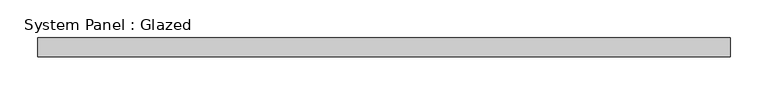
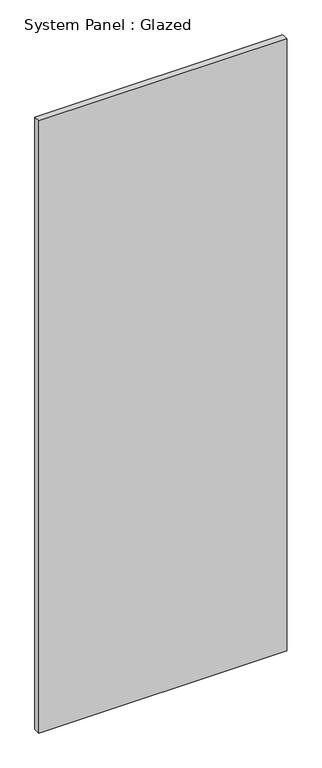
"""IFC4 building model written with IfcOpenShell, lengths in millimetres: plate geometry, System Panel : Glazed."""

from ifc_helpers import new_model, si_unit, origin, origin_with_axes, place, context, project, spatial, polyline, outline, extrude, source, transform, mapped, element, save


def system_panel_glazed_003a5872(model_context):
    return source(origin(), model_context, "Body", "SweptSolid", [
        extrude(outline(polyline([(460.375, 19.05), (-460.375, 19.05), (-460.375, 44.45), (460.375, 44.45), (460.375, 19.05)])), origin_with_axes(), (0.0, 0.0, 1.0), 2402.4963211),
    ])


if __name__ == "__main__":
    model = new_model("IFC4")
    model_context = context("Model", 3, world=origin())
    ifc_project = project(units=[si_unit("LENGTHUNIT", "METRE", prefix="MILLI")], contexts=[model_context])
    site = spatial("IfcSite", under=ifc_project)
    building = spatial("IfcBuilding", under=site)
    placement = place(None, origin())
    system_panel_glazed_shape = system_panel_glazed_003a5872(model_context)
    element("IfcPlate", 1, ObjectType="System Panel : Glazed", at=placement, inside=building, context=model_context, shape_type="MappedRepresentation", body=[
        mapped(system_panel_glazed_shape, transform((0.0, 0.0, 0.0), x_axis=(1.0, 0.0, 0.0), y_axis=(0.0, 1.0, 0.0), z_axis=(0.0, 0.0, 1.0))),
    ])
    save(model, "model.ifc")

# Revit data of these elements
# Type "System Panel : Glazed"
#   Construction Type Id = "GSP4R"
#   Analytic Construction = "1/8 in Pilkington single glazing"
#   Visual Light Transmittance = 0.9
#   Solar Heat Gain Coefficient = 0.86
#   Heat Transfer Coefficient (U) = 1.18115 BTU/(h·ft²·°F)
#   Define Thermal Properties by = 1
# Element 1 (IfcPlate, "System Panel : Glazed")
#   Materials on its faces: "Glass"
# Materials
#   "Glass": class "Glass", colour RGB 0 128 192, transparency 0.75, Description = "Soda Lime Glass", Cost = 0
